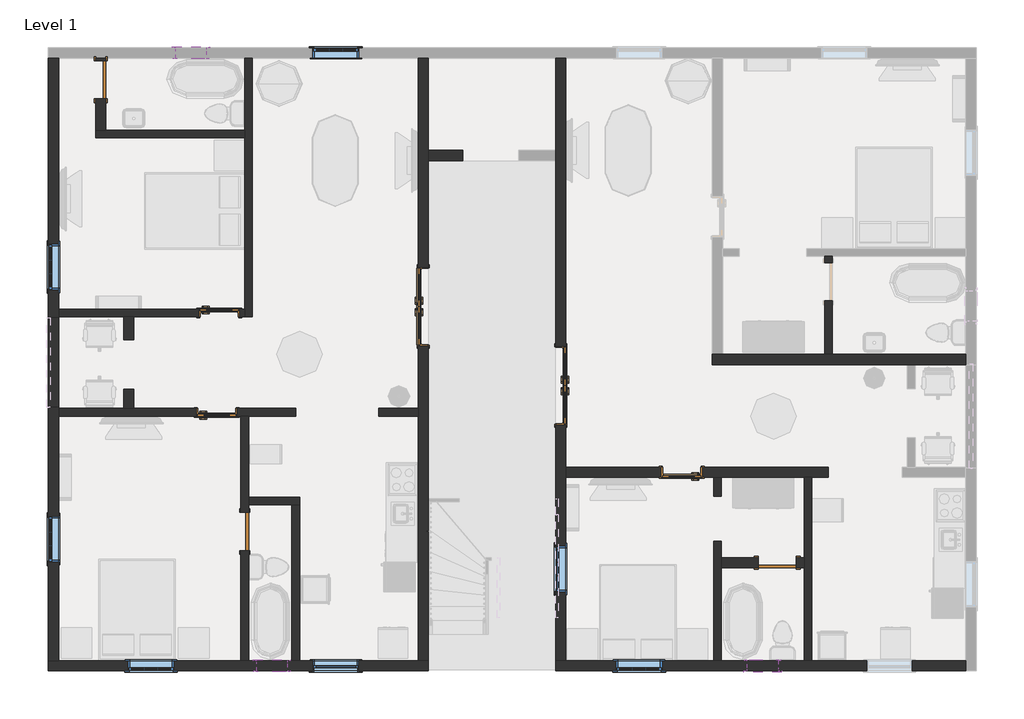
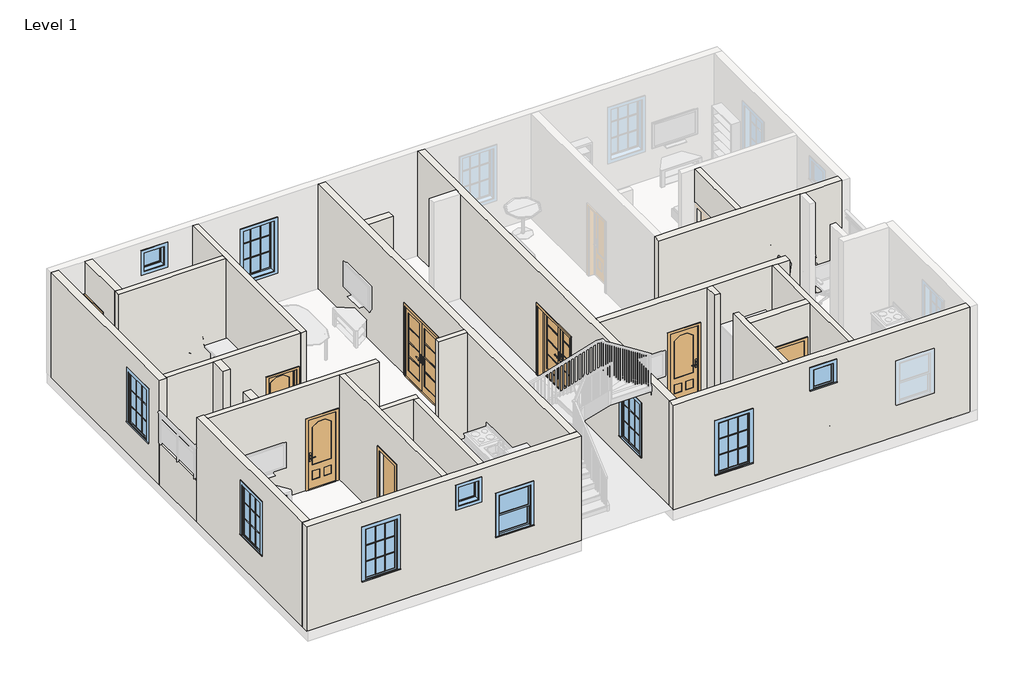
# One storey, part 1 of 4: 26 walls, 10 windows, 8 doors.
"""IFC4 building model written with IfcOpenShell, lengths in millimetres."""

from ifc_helpers import new_model, si_unit, frame, origin, origin_with_axes, place, context, project, spatial, polyline, outline, extrude, faceted_brep, transform, mapped, element, save
from components import door_4b146b56, door_14b9be53, door_41326d50, door_b03bd389, door_53b1b562, door_255cab33, window_58e1470a, window_31198920, window_e41d21a6

model = new_model("IFC4")

# Units and contexts
model_context = context("Model", 3, world=origin())
ifc_project = project(units=[si_unit("LENGTHUNIT", "METRE", prefix="MILLI")], contexts=[model_context])

# Site, building, storey
site = spatial("IfcSite", under=ifc_project)
building = spatial("IfcBuilding", under=site)
storey = spatial("IfcBuildingStorey", under=building, Name="Level 1", Elevation=0.0)

# Doors
placement = place(None, origin())
door_shape = door_4b146b56(model_context)
element("IfcDoor", 1, ObjectType="30\" x 80\"", at=placement, inside=storey, context=model_context, shape_type="MappedRepresentation", body=[
    mapped(door_shape, transform((-13233.5808972, 7613.5673354, 0.0), x_axis=(-1.0, 0.0, 0.0), y_axis=(0.0, -1.0, 0.0), z_axis=(0.0, 0.0, 1.0))),
])
door_2_shape = door_14b9be53(model_context)
element("IfcDoor", 2, ObjectType="30\" x 80\"", at=placement, inside=storey, context=model_context, shape_type="MappedRepresentation", body=[
    mapped(door_2_shape, transform((-13284.3808972, 5626.0173354, 0.0), x_axis=(-1.0, 0.0, 0.0), y_axis=(0.0, -1.0, 0.0), z_axis=(0.0, 0.0, 1.0))),
])
door_3_shape = door_41326d50(model_context)
element("IfcDoor", 3, ObjectType="30\" x 80\"", at=placement, inside=storey, context=model_context, shape_type="MappedRepresentation", body=[
    mapped(door_3_shape, transform((-4013.3808972, 4432.2173354, 0.0), x_axis=(1.0, 0.0, 0.0), y_axis=(0.0, 1.0, 0.0), z_axis=(0.0, 0.0, 1.0))),
])
door_4_shape = door_b03bd389(model_context)
element("IfcDoor", 4, ObjectType="Door-Exterior-Double-Full Glass-Wood_Clad : 60\" x 80\"", at=placement, inside=storey, context=model_context, shape_type="MappedRepresentation", body=[
    mapped(door_4_shape, transform((-9172.7558972, 7737.3923354, 0.0), x_axis=(0.0, 1.0, 0.0), y_axis=(-1.0, 0.0, 0.0), z_axis=(0.0, 0.0, 1.0))),
])
element("IfcDoor", 5, ObjectType="Door-Exterior-Double-Full Glass-Wood_Clad : 60\" x 80\"", at=placement, inside=storey, context=model_context, shape_type="MappedRepresentation", body=[
    mapped(door_4_shape, transform((-6423.2058972, 6162.5923354, 0.0), x_axis=(0.0, -1.0, 0.0), y_axis=(1.0, 0.0, 0.0), z_axis=(0.0, 0.0, 1.0))),
])
door_5_shape = door_53b1b562(model_context)
element("IfcDoor", 6, ObjectType="Single-Flush : 30\" x 80\"", at=placement, inside=storey, context=model_context, shape_type="MappedRepresentation", body=[
    mapped(door_5_shape, transform((-15595.7808972, 12258.5923354, 0.0), x_axis=(0.0, 1.0, 0.0), y_axis=(-1.0, 0.0, 0.0), z_axis=(0.0, 0.0, 1.0))),
])
element("IfcDoor", 7, ObjectType="Single-Flush : 30\" x 80\"", at=placement, inside=storey, context=model_context, shape_type="MappedRepresentation", body=[
    mapped(door_5_shape, transform((-2108.3808972, 2631.9923354, 0.0), x_axis=(1.0, 0.0, 0.0), y_axis=(0.0, 1.0, 0.0), z_axis=(0.0, 0.0, 1.0))),
])
door_6_shape = door_255cab33(model_context)
element("IfcDoor", 8, ObjectType="Single-Flush : 30\" x 80\"", at=placement, inside=storey, context=model_context, shape_type="MappedRepresentation", body=[
    mapped(door_6_shape, transform((-12725.5808972, 3254.2923354, 0.0), x_axis=(0.0, 1.0, 0.0), y_axis=(-1.0, 0.0, 0.0), z_axis=(0.0, 0.0, 1.0))),
])

# Walls
element("IfcWall", 9, ObjectType="Generic - 8\"", at=placement, inside=storey, context=model_context, shape_type="Brep", body=[
    faceted_brep([(1650.8191028, 676.1923354, 0.0), (-1422.5808972, 676.1923354, 0.0), (-1574.9808972, 676.1923354, 0.0), (-3225.9808972, 676.1923354, 0.0), (-3378.3808972, 676.1923354, 0.0), (-6324.7808972, 676.1923354, 0.0), (-6527.9808972, 676.1923354, 0.0), (-6527.9808972, 676.1923354, 3048.0), (-6324.7808972, 676.1923354, 3048.0), (-3378.3808972, 676.1923354, 3048.0), (-3225.9808972, 676.1923354, 3048.0), (-1574.9808972, 676.1923354, 3048.0), (-1422.5808972, 676.1923354, 3048.0), (1650.8191028, 676.1923354, 3048.0), (-330.3808972, 676.1923354, 2133.6), (-330.3808972, 676.1923354, 914.4), (584.0191028, 676.1923354, 914.4), (584.0191028, 676.1923354, 2133.6), (-5321.4808972, 676.1923354, 2133.6), (-5321.4808972, 676.1923354, 609.6), (-4407.0808972, 676.1923354, 609.6), (-4407.0808972, 676.1923354, 2133.6), (-2705.2808972, 676.1923354, 2768.6), (-2705.2808972, 676.1923354, 2159.0), (-2095.6808972, 676.1923354, 2159.0), (-2095.6808972, 676.1923354, 2768.6), (1650.8191028, 472.9923354, 0.0), (1650.8191028, 472.9923354, 3048.0), (-6527.9808972, 472.9923354, 3048.0), (-6527.9808972, 472.9923354, 0.0), (-330.3808972, 472.9923354, 2133.6), (584.0191028, 472.9923354, 2133.6), (584.0191028, 472.9923354, 914.4), (-330.3808972, 472.9923354, 914.4), (-5321.4808972, 472.9923354, 2133.6), (-4407.0808972, 472.9923354, 2133.6), (-4407.0808972, 472.9923354, 609.6), (-5321.4808972, 472.9923354, 609.6), (-2705.2808972, 472.9923354, 2768.6), (-2095.6808972, 472.9923354, 2768.6), (-2095.6808972, 472.9923354, 2159.0), (-2705.2808972, 472.9923354, 2159.0)], [[[0, 1, 2, 3, 4, 5, 6, 7, 8, 9, 10, 11, 12, 13], [14, 15, 16, 17], [18, 19, 20, 21], [22, 23, 24, 25]], [[26, 27, 28, 29], [30, 31, 32, 33], [34, 35, 36, 37], [38, 39, 40, 41]], [[6, 5, 4, 3, 2, 1, 0, 26, 29]], [[13, 12, 11, 10, 9, 8, 7, 28, 27]], [[0, 13, 27, 26]], [[7, 6, 29, 28]], [[15, 14, 30, 33]], [[16, 15, 33, 32]], [[17, 16, 32, 31]], [[14, 17, 31, 30]], [[19, 18, 34, 37]], [[20, 19, 37, 36]], [[21, 20, 36, 35]], [[18, 21, 35, 34]], [[23, 22, 38, 41]], [[24, 23, 41, 40]], [[25, 24, 40, 39]], [[22, 25, 39, 38]]]),
])
element("IfcWall", 10, ObjectType="Generic - 8\"", at=placement, inside=storey, context=model_context, shape_type="Brep", body=[
    faceted_brep([(-16433.9808972, 676.1923354, 0.0), (-16433.9808972, 5552.9923354, 0.0), (-16433.9808972, 5705.3923354, 0.0), (-16433.9808972, 5730.7923354, 0.0), (-16433.9808972, 5730.7923354, 1219.2), (-16433.9808972, 5730.7923354, 3048.0), (-16433.9808972, 5705.3923354, 3048.0), (-16433.9808972, 5552.9923354, 3048.0), (-16433.9808972, 676.1923354, 3048.0), (-16433.9808972, 3559.0923354, 2438.4), (-16433.9808972, 3559.0923354, 914.4), (-16433.9808972, 2644.6923354, 914.4), (-16433.9808972, 2644.6923354, 2438.4), (-16637.1808972, 676.1923354, 0.0), (-16637.1808972, 676.1923354, 3048.0), (-16637.1808972, 5730.7923354, 3048.0), (-16637.1808972, 5730.7923354, 1219.2), (-16637.1808972, 5730.7923354, 0.0), (-16637.1808972, 3559.0923354, 2438.4), (-16637.1808972, 2644.6923354, 2438.4), (-16637.1808972, 2644.6923354, 914.4), (-16637.1808972, 3559.0923354, 914.4)], [[[0, 1, 2, 3, 4, 5, 6, 7, 8], [9, 10, 11, 12]], [[13, 14, 15, 16, 17], [18, 19, 20, 21]], [[3, 2, 1, 0, 13, 17]], [[5, 4, 3, 17, 16, 15]], [[8, 7, 6, 5, 15, 14]], [[0, 8, 14, 13]], [[10, 9, 18, 21]], [[11, 10, 21, 20]], [[12, 11, 20, 19]], [[9, 12, 19, 18]]]),
])
element("IfcWall", 11, ObjectType="Generic - 8\"", at=placement, inside=storey, context=model_context, shape_type="Brep", body=[
    faceted_brep([(-6527.9808972, 676.1923354, 3048.0), (-6527.9808972, 10645.6923354, 3048.0), (-6527.9808972, 10848.8923354, 3048.0), (-6527.9808972, 12690.3923354, 3048.0), (-6527.9808972, 12690.3923354, 0.0), (-6527.9808972, 10848.8923354, 0.0), (-6527.9808972, 10645.6923354, 0.0), (-6527.9808972, 6949.9923354, 0.0), (-6527.9808972, 6949.9923354, 2057.4), (-6527.9808972, 5375.1923354, 2057.4), (-6527.9808972, 5375.1923354, 0.0), (-6527.9808972, 676.1923354, 0.0), (-6527.9808972, 2962.1923354, 2133.6), (-6527.9808972, 2047.7923354, 2133.6), (-6527.9808972, 2047.7923354, 609.6), (-6527.9808972, 2962.1923354, 609.6), (-6324.7808972, 12690.3923354, 3048.0), (-6324.7808972, 4536.9923354, 3048.0), (-6324.7808972, 4333.7923354, 3048.0), (-6324.7808972, 676.1923354, 3048.0), (-6324.7808972, 676.1923354, 0.0), (-6324.7808972, 4333.7923354, 0.0), (-6324.7808972, 4536.9923354, 0.0), (-6324.7808972, 5375.1923354, 0.0), (-6324.7808972, 5375.1923354, 2057.4), (-6324.7808972, 6949.9923354, 2057.4), (-6324.7808972, 6949.9923354, 0.0), (-6324.7808972, 12690.3923354, 0.0), (-6324.7808972, 2962.1923354, 2133.6), (-6324.7808972, 2962.1923354, 609.6), (-6324.7808972, 2047.7923354, 609.6), (-6324.7808972, 2047.7923354, 2133.6)], [[[0, 1, 2, 3, 4, 5, 6, 7, 8, 9, 10, 11], [12, 13, 14, 15]], [[16, 17, 18, 19, 20, 21, 22, 23, 24, 25, 26, 27], [28, 29, 30, 31]], [[4, 27, 26, 7, 6, 5]], [[20, 11, 10, 23, 22, 21]], [[3, 2, 1, 0, 19, 18, 17, 16]], [[4, 3, 16, 27]], [[0, 11, 20, 19]], [[9, 24, 23, 10]], [[24, 9, 8, 25]], [[25, 8, 7, 26]], [[29, 28, 12, 15]], [[30, 29, 15, 14]], [[31, 30, 14, 13]], [[28, 31, 13, 12]]]),
])
element("IfcWall", 12, ObjectType="Generic - 8\"", at=placement, inside=storey, context=model_context, shape_type="Brep", body=[
    faceted_brep([(-9271.1808972, 676.1923354, 3048.0), (-9271.1808972, 5552.9923354, 3048.0), (-9271.1808972, 5705.3923354, 3048.0), (-9271.1808972, 12690.3923354, 3048.0), (-9271.1808972, 12690.3923354, 0.0), (-9271.1808972, 8524.7923354, 0.0), (-9271.1808972, 8524.7923354, 2057.4), (-9271.1808972, 6949.9923354, 2057.4), (-9271.1808972, 6949.9923354, 0.0), (-9271.1808972, 5705.3923354, 0.0), (-9271.1808972, 5552.9923354, 0.0), (-9271.1808972, 676.1923354, 0.0), (-9067.9808972, 12690.3923354, 3048.0), (-9067.9808972, 10848.8923354, 3048.0), (-9067.9808972, 10645.6923354, 3048.0), (-9067.9808972, 676.1923354, 3048.0), (-9067.9808972, 676.1923354, 0.0), (-9067.9808972, 6949.9923354, 0.0), (-9067.9808972, 6949.9923354, 2057.4), (-9067.9808972, 8524.7923354, 2057.4), (-9067.9808972, 8524.7923354, 0.0), (-9067.9808972, 10645.6923354, 0.0), (-9067.9808972, 10848.8923354, 0.0), (-9067.9808972, 12690.3923354, 0.0)], [[[0, 1, 2, 3, 4, 5, 6, 7, 8, 9, 10, 11]], [[12, 13, 14, 15, 16, 17, 18, 19, 20, 21, 22, 23]], [[4, 23, 22, 21, 20, 5]], [[16, 11, 10, 9, 8, 17]], [[3, 2, 1, 0, 15, 14, 13, 12]], [[4, 3, 12, 23]], [[0, 11, 16, 15]], [[19, 6, 5, 20]], [[6, 19, 18, 7]], [[7, 18, 17, 8]]]),
])
element("IfcWall", 13, ObjectType="Generic - 8\"", at=placement, inside=storey, context=model_context, shape_type="Brep", body=[
    faceted_brep([(-1092.3808972, 4333.7923354, 0.0), (-1092.3808972, 4333.7923354, 3048.0), (-1422.5808972, 4333.7923354, 3048.0), (-1574.9808972, 4333.7923354, 3048.0), (-3225.9808972, 4333.7923354, 3048.0), (-3378.3808972, 4333.7923354, 3048.0), (-6324.7808972, 4333.7923354, 3048.0), (-6324.7808972, 4333.7923354, 0.0), (-4419.7808972, 4333.7923354, 0.0), (-4419.7808972, 4333.7923354, 2057.4), (-3606.9808972, 4333.7923354, 2057.4), (-3606.9808972, 4333.7923354, 0.0), (-3378.3808972, 4333.7923354, 0.0), (-3225.9808972, 4333.7923354, 0.0), (-1574.9808972, 4333.7923354, 0.0), (-1422.5808972, 4333.7923354, 0.0), (-1092.3808972, 4536.9923354, 3048.0), (-1092.3808972, 4536.9923354, 0.0), (-3606.9808972, 4536.9923354, 0.0), (-3606.9808972, 4536.9923354, 2057.4), (-4419.7808972, 4536.9923354, 2057.4), (-4419.7808972, 4536.9923354, 0.0), (-6324.7808972, 4536.9923354, 0.0), (-6324.7808972, 4536.9923354, 3048.0)], [[[0, 1, 2, 3, 4, 5, 6, 7, 8, 9, 10, 11, 12, 13, 14, 15]], [[16, 17, 18, 19, 20, 21, 22, 23]], [[17, 0, 15, 14, 13, 12, 11, 18]], [[7, 22, 21, 8]], [[1, 0, 17, 16]], [[6, 5, 4, 3, 2, 1, 16, 23]], [[7, 6, 23, 22]], [[10, 19, 18, 11]], [[19, 10, 9, 20]], [[20, 9, 8, 21]]]),
])
element("IfcWall", 14, ObjectType="Generic - 8\"", at=placement, inside=storey, context=model_context, shape_type="Brep", body=[
    faceted_brep([(1650.8191028, 6784.8923354, 0.0), (-1016.1808972, 6784.8923354, 0.0), (-1168.5808972, 6784.8923354, 0.0), (-3200.5808972, 6784.8923354, 0.0), (-3403.7808972, 6784.8923354, 0.0), (-3403.7808972, 6784.8923354, 3048.0), (-3200.5808972, 6784.8923354, 3048.0), (-1168.5808972, 6784.8923354, 3048.0), (-1016.1808972, 6784.8923354, 3048.0), (1650.8191028, 6784.8923354, 3048.0), (1650.8191028, 6581.6923354, 0.0), (1650.8191028, 6581.6923354, 3048.0), (634.8191028, 6581.6923354, 3048.0), (482.4191028, 6581.6923354, 3048.0), (-3403.7808972, 6581.6923354, 3048.0), (-3403.7808972, 6581.6923354, 0.0), (482.4191028, 6581.6923354, 0.0), (634.8191028, 6581.6923354, 0.0)], [[[0, 1, 2, 3, 4, 5, 6, 7, 8, 9]], [[10, 11, 12, 13, 14, 15, 16, 17]], [[4, 3, 2, 1, 0, 10, 17, 16, 15]], [[9, 8, 7, 6, 5, 14, 13, 12, 11]], [[0, 9, 11, 10]], [[5, 4, 15, 14]]]),
])
element("IfcWall", 15, ObjectType="Generic - 8\"", at=placement, inside=storey, context=model_context, shape_type="SweptSolid", body=[
    extrude(outline(polyline([(-8382.1808972, 10645.6923354), (-9067.9808972, 10645.6923354), (-9067.9808972, 10848.8923354), (-8382.1808972, 10848.8923354), (-8382.1808972, 10645.6923354)])), origin_with_axes(), (0.0, 0.0, 1.0), 3048.0),
])
element("IfcWall", 16, ObjectType="Generic - 8\"", at=placement, inside=storey, context=model_context, shape_type="Brep", body=[
    faceted_brep([(-9067.9808972, 676.1923354, 0.0), (-9271.1808972, 676.1923354, 0.0), (-11633.3808972, 676.1923354, 0.0), (-11785.7808972, 676.1923354, 0.0), (-12649.3808972, 676.1923354, 0.0), (-12801.7808972, 676.1923354, 0.0), (-16433.9808972, 676.1923354, 0.0), (-16637.1808972, 676.1923354, 0.0), (-16637.1808972, 676.1923354, 3048.0), (-16433.9808972, 676.1923354, 3048.0), (-12801.7808972, 676.1923354, 3048.0), (-12649.3808972, 676.1923354, 3048.0), (-11785.7808972, 676.1923354, 3048.0), (-11633.3808972, 676.1923354, 3048.0), (-9271.1808972, 676.1923354, 3048.0), (-9067.9808972, 676.1923354, 3048.0), (-15049.6808972, 676.1923354, 2438.4), (-15049.6808972, 676.1923354, 914.4), (-14135.2808972, 676.1923354, 914.4), (-14135.2808972, 676.1923354, 2438.4), (-11366.6808972, 676.1923354, 2133.6), (-11366.6808972, 676.1923354, 914.4), (-10452.2808972, 676.1923354, 914.4), (-10452.2808972, 676.1923354, 2133.6), (-11874.6808972, 676.1923354, 2768.6), (-12484.2808972, 676.1923354, 2768.6), (-12484.2808972, 676.1923354, 2159.0), (-11874.6808972, 676.1923354, 2159.0), (-9067.9808972, 472.9923354, 0.0), (-9067.9808972, 472.9923354, 3048.0), (-16637.1808972, 472.9923354, 3048.0), (-16637.1808972, 472.9923354, 0.0), (-15049.6808972, 472.9923354, 2438.4), (-14135.2808972, 472.9923354, 2438.4), (-14135.2808972, 472.9923354, 914.4), (-15049.6808972, 472.9923354, 914.4), (-11366.6808972, 472.9923354, 2133.6), (-10452.2808972, 472.9923354, 2133.6), (-10452.2808972, 472.9923354, 914.4), (-11366.6808972, 472.9923354, 914.4), (-11874.6808972, 472.9923354, 2768.6), (-11874.6808972, 472.9923354, 2159.0), (-12484.2808972, 472.9923354, 2159.0), (-12484.2808972, 472.9923354, 2768.6)], [[[0, 1, 2, 3, 4, 5, 6, 7, 8, 9, 10, 11, 12, 13, 14, 15], [16, 17, 18, 19], [20, 21, 22, 23], [24, 25, 26, 27]], [[28, 29, 30, 31], [32, 33, 34, 35], [36, 37, 38, 39], [40, 41, 42, 43]], [[7, 6, 5, 4, 3, 2, 1, 0, 28, 31]], [[15, 14, 13, 12, 11, 10, 9, 8, 30, 29]], [[8, 7, 31, 30]], [[0, 15, 29, 28]], [[17, 16, 32, 35]], [[18, 17, 35, 34]], [[19, 18, 34, 33]], [[16, 19, 33, 32]], [[21, 20, 36, 39]], [[22, 21, 39, 38]], [[23, 22, 38, 37]], [[20, 23, 37, 36]], [[41, 40, 24, 27]], [[42, 41, 27, 26]], [[43, 42, 26, 25]], [[40, 43, 25, 24]]]),
])
element("IfcWall", 17, ObjectType="Generic - 8\"", at=placement, inside=storey, context=model_context, shape_type="SweptSolid", body=[
    extrude(outline(polyline([(12690.3923354, 0.0), (12639.5923354, 0.0), (12639.5923354, 2032.0), (11877.5923354, 2032.0), (11877.5923354, 0.0), (11255.2923354, 0.0), (11255.2923354, 3048.0), (12690.3923354, 3048.0), (12690.3923354, 0.0)])), frame((-15697.3808972, 0.0, 0.0), z_axis=(1.0, 0.0, 0.0), x_axis=(0.0, 1.0, 0.0)), (0.0, 0.0, 1.0), 203.2),
])
element("IfcWall", 18, ObjectType="Generic - 8\"", at=placement, inside=storey, context=model_context, shape_type="SweptSolid", body=[
    extrude(outline(polyline([(2032.0, -1727.3808972), (0.0, -1727.3808972), (0.0, -1574.9808972), (3048.0, -1574.9808972), (3048.0, -3225.9808972), (0.0, -3225.9808972), (0.0, -2489.3808972), (2032.0, -2489.3808972), (2032.0, -1727.3808972)])), frame((0.0, 2530.3923354, 0.0), z_axis=(0.0, 1.0, 0.0), x_axis=(0.0, 0.0, 1.0)), (0.0, 0.0, 1.0), 203.2),
])
element("IfcWall", 19, ObjectType="Generic - 8\"", at=placement, inside=storey, context=model_context, shape_type="SweptSolid", body=[
    extrude(outline(polyline([(-15138.5808972, 7076.9923354), (-15138.5808972, 7534.1923354), (-14935.3808972, 7534.1923354), (-14935.3808972, 7076.9923354), (-15138.5808972, 7076.9923354)])), origin_with_axes(), (0.0, 0.0, 1.0), 3048.0),
])
element("IfcWall", 20, ObjectType="Generic - 8\"", at=placement, inside=storey, context=model_context, shape_type="SweptSolid", body=[
    extrude(outline(polyline([(-15138.5808972, 5705.3923354), (-15138.5808972, 6086.3923354), (-14935.3808972, 6086.3923354), (-14935.3808972, 5705.3923354), (-15138.5808972, 5705.3923354)])), origin_with_axes(), (0.0, 0.0, 1.0), 3048.0),
])
element("IfcWall", 21, ObjectType="Generic - 8\"", at=placement, inside=storey, context=model_context, shape_type="Brep", body=[
    faceted_brep([(-16433.9808972, 7508.7923354, 0.0), (-16433.9808972, 7534.1923354, 0.0), (-16433.9808972, 7686.5923354, 0.0), (-16433.9808972, 12690.3923354, 0.0), (-16433.9808972, 12690.3923354, 3048.0), (-16433.9808972, 7686.5923354, 3048.0), (-16433.9808972, 7534.1923354, 3048.0), (-16433.9808972, 7508.7923354, 3048.0), (-16433.9808972, 7508.7923354, 1219.2), (-16433.9808972, 8981.9923354, 2438.4), (-16433.9808972, 8981.9923354, 914.4), (-16433.9808972, 8067.5923354, 914.4), (-16433.9808972, 8067.5923354, 2438.4), (-16637.1808972, 7508.7923354, 0.0), (-16637.1808972, 7508.7923354, 1219.2), (-16637.1808972, 7508.7923354, 3048.0), (-16637.1808972, 12690.3923354, 3048.0), (-16637.1808972, 12690.3923354, 0.0), (-16637.1808972, 8981.9923354, 2438.4), (-16637.1808972, 8067.5923354, 2438.4), (-16637.1808972, 8067.5923354, 914.4), (-16637.1808972, 8981.9923354, 914.4)], [[[0, 1, 2, 3, 4, 5, 6, 7, 8], [9, 10, 11, 12]], [[13, 14, 15, 16, 17], [18, 19, 20, 21]], [[3, 2, 1, 0, 13, 17]], [[7, 6, 5, 4, 16, 15]], [[0, 8, 7, 15, 14, 13]], [[4, 3, 17, 16]], [[10, 9, 18, 21]], [[11, 10, 21, 20]], [[12, 11, 20, 19]], [[9, 12, 19, 18]]]),
])
element("IfcWall", 22, ObjectType="Generic - 8\"", at=placement, inside=storey, context=model_context, shape_type="SweptSolid", body=[
    extrude(outline(polyline([(-16433.9808972, 7508.7923354), (-16433.9808972, 5730.7923354), (-16637.1808972, 5730.7923354), (-16637.1808972, 7508.7923354), (-16433.9808972, 7508.7923354)])), origin_with_axes(), (0.0, 0.0, 1.0), 1219.2),
])
element("IfcWall", 23, ObjectType="INNER", at=placement, inside=storey, context=model_context, shape_type="Brep", body=[
    faceted_brep([(-12725.5808972, 12690.3923354, 0.0), (-12725.5808972, 11255.2923354, 0.0), (-12725.5808972, 11102.8923354, 0.0), (-12725.5808972, 7686.5923354, 0.0), (-12725.5808972, 7534.1923354, 0.0), (-12725.5808972, 7534.1923354, 3048.0), (-12725.5808972, 7686.5923354, 3048.0), (-12725.5808972, 11102.8923354, 3048.0), (-12725.5808972, 11255.2923354, 3048.0), (-12725.5808972, 12690.3923354, 3048.0), (-12573.1808972, 12690.3923354, 0.0), (-12573.1808972, 12690.3923354, 3048.0), (-12573.1808972, 7534.1923354, 3048.0), (-12573.1808972, 7534.1923354, 0.0)], [[[0, 1, 2, 3, 4, 5, 6, 7, 8, 9]], [[10, 11, 12, 13]], [[4, 3, 2, 1, 0, 10, 13]], [[9, 8, 7, 6, 5, 12, 11]], [[0, 9, 11, 10]], [[5, 4, 13, 12]]]),
])
element("IfcWall", 24, ObjectType="INNER", at=placement, inside=storey, context=model_context, shape_type="SweptSolid", body=[
    extrude(outline(polyline([(-10058.5808972, 5705.3923354), (-9271.1808972, 5705.3923354), (-9271.1808972, 5552.9923354), (-10058.5808972, 5552.9923354), (-10058.5808972, 5705.3923354)])), origin_with_axes(), (0.0, 0.0, 1.0), 3048.0),
])
element("IfcWall", 25, ObjectType="INNER", at=placement, inside=storey, context=model_context, shape_type="Brep", body=[
    faceted_brep([(-12725.5808972, 7534.1923354, 3048.0), (-14935.3808972, 7534.1923354, 3048.0), (-15138.5808972, 7534.1923354, 3048.0), (-16433.9808972, 7534.1923354, 3048.0), (-16433.9808972, 7534.1923354, 0.0), (-15138.5808972, 7534.1923354, 0.0), (-14935.3808972, 7534.1923354, 0.0), (-13639.9808972, 7534.1923354, 0.0), (-13639.9808972, 7534.1923354, 2057.4), (-12827.1808972, 7534.1923354, 2057.4), (-12827.1808972, 7534.1923354, 0.0), (-12725.5808972, 7534.1923354, 0.0), (-16433.9808972, 7686.5923354, 3048.0), (-12725.5808972, 7686.5923354, 3048.0), (-12725.5808972, 7686.5923354, 0.0), (-12827.1808972, 7686.5923354, 0.0), (-12827.1808972, 7686.5923354, 2057.4), (-13639.9808972, 7686.5923354, 2057.4), (-13639.9808972, 7686.5923354, 0.0), (-16433.9808972, 7686.5923354, 0.0)], [[[0, 1, 2, 3, 4, 5, 6, 7, 8, 9, 10, 11]], [[12, 13, 14, 15, 16, 17, 18, 19]], [[4, 19, 18, 7, 6, 5]], [[14, 11, 10, 15]], [[3, 2, 1, 0, 13, 12]], [[4, 3, 12, 19]], [[0, 11, 14, 13]], [[17, 8, 7, 18]], [[8, 17, 16, 9]], [[9, 16, 15, 10]]]),
])
element("IfcWall", 26, ObjectType="INNER", at=placement, inside=storey, context=model_context, shape_type="Brep", body=[
    faceted_brep([(-12801.7808972, 5552.9923354, 0.0), (-12801.7808972, 3635.2923354, 0.0), (-12801.7808972, 3635.2923354, 2032.0), (-12801.7808972, 2873.2923354, 2032.0), (-12801.7808972, 2873.2923354, 0.0), (-12801.7808972, 676.1923354, 0.0), (-12801.7808972, 676.1923354, 3048.0), (-12801.7808972, 5552.9923354, 3048.0), (-12649.3808972, 3635.2923354, 2032.0), (-12649.3808972, 3635.2923354, 0.0), (-12649.3808972, 3787.6923354, 0.0), (-12649.3808972, 3940.0923354, 0.0), (-12649.3808972, 5552.9923354, 0.0), (-12649.3808972, 5552.9923354, 3048.0), (-12649.3808972, 3940.0923354, 3048.0), (-12649.3808972, 3787.6923354, 3048.0), (-12649.3808972, 676.1923354, 3048.0), (-12649.3808972, 676.1923354, 0.0), (-12649.3808972, 2873.2923354, 0.0), (-12649.3808972, 2873.2923354, 2032.0)], [[[0, 1, 2, 3, 4, 5, 6, 7]], [[8, 9, 10, 11, 12, 13, 14, 15, 16, 17, 18, 19]], [[18, 17, 5, 4]], [[12, 11, 10, 9, 1, 0]], [[7, 6, 16, 15, 14, 13]], [[6, 5, 17, 16]], [[0, 7, 13, 12]], [[2, 1, 9, 8]], [[3, 2, 8, 19]], [[4, 3, 19, 18]]]),
])
element("IfcWall", 27, ObjectType="INNER", at=placement, inside=storey, context=model_context, shape_type="Brep", body=[
    faceted_brep([(-16433.9808972, 5705.3923354, 3048.0), (-15138.5808972, 5705.3923354, 3048.0), (-14935.3808972, 5705.3923354, 3048.0), (-11709.5808972, 5705.3923354, 3048.0), (-11709.5808972, 5705.3923354, 0.0), (-12877.9808972, 5705.3923354, 0.0), (-12877.9808972, 5705.3923354, 2057.4), (-13690.7808972, 5705.3923354, 2057.4), (-13690.7808972, 5705.3923354, 0.0), (-14935.3808972, 5705.3923354, 0.0), (-15138.5808972, 5705.3923354, 0.0), (-16433.9808972, 5705.3923354, 0.0), (-11709.5808972, 5552.9923354, 3048.0), (-12649.3808972, 5552.9923354, 3048.0), (-12801.7808972, 5552.9923354, 3048.0), (-16433.9808972, 5552.9923354, 3048.0), (-16433.9808972, 5552.9923354, 0.0), (-13690.7808972, 5552.9923354, 0.0), (-13690.7808972, 5552.9923354, 2057.4), (-12877.9808972, 5552.9923354, 2057.4), (-12877.9808972, 5552.9923354, 0.0), (-12801.7808972, 5552.9923354, 0.0), (-12649.3808972, 5552.9923354, 0.0), (-11709.5808972, 5552.9923354, 0.0)], [[[0, 1, 2, 3, 4, 5, 6, 7, 8, 9, 10, 11]], [[12, 13, 14, 15, 16, 17, 18, 19, 20, 21, 22, 23]], [[4, 23, 22, 21, 20, 5]], [[16, 11, 10, 9, 8, 17]], [[3, 2, 1, 0, 15, 14, 13, 12]], [[4, 3, 12, 23]], [[0, 11, 16, 15]], [[7, 18, 17, 8]], [[18, 7, 6, 19]], [[19, 6, 5, 20]]]),
])
element("IfcWall", 28, ObjectType="INNER", at=placement, inside=storey, context=model_context, shape_type="Brep", body=[
    faceted_brep([(-1574.9808972, 4333.7923354, 0.0), (-1574.9808972, 2733.5923354, 0.0), (-1574.9808972, 2530.3923354, 0.0), (-1574.9808972, 676.1923354, 0.0), (-1574.9808972, 676.1923354, 3048.0), (-1574.9808972, 2530.3923354, 3048.0), (-1574.9808972, 2733.5923354, 3048.0), (-1574.9808972, 4333.7923354, 3048.0), (-1422.5808972, 4333.7923354, 0.0), (-1422.5808972, 4333.7923354, 3048.0), (-1422.5808972, 676.1923354, 3048.0), (-1422.5808972, 676.1923354, 0.0)], [[[0, 1, 2, 3, 4, 5, 6, 7]], [[8, 9, 10, 11]], [[3, 2, 1, 0, 8, 11]], [[7, 6, 5, 4, 10, 9]], [[4, 3, 11, 10]], [[0, 7, 9, 8]]]),
])
element("IfcWall", 29, ObjectType="INNER", at=placement, inside=storey, context=model_context, shape_type="Brep", body=[
    faceted_brep([(-3225.9808972, 676.1923354, 0.0), (-3225.9808972, 2530.3923354, 0.0), (-3225.9808972, 2733.5923354, 0.0), (-3225.9808972, 3063.7923354, 0.0), (-3225.9808972, 3063.7923354, 3048.0), (-3225.9808972, 2733.5923354, 3048.0), (-3225.9808972, 2530.3923354, 3048.0), (-3225.9808972, 676.1923354, 3048.0), (-3378.3808972, 676.1923354, 0.0), (-3378.3808972, 676.1923354, 3048.0), (-3378.3808972, 3063.7923354, 3048.0), (-3378.3808972, 3063.7923354, 0.0)], [[[0, 1, 2, 3, 4, 5, 6, 7]], [[8, 9, 10, 11]], [[3, 2, 1, 0, 8, 11]], [[4, 3, 11, 10]], [[7, 6, 5, 4, 10, 9]], [[0, 7, 9, 8]]]),
])
element("IfcWall", 30, ObjectType="INNER", at=placement, inside=storey, context=model_context, shape_type="SweptSolid", body=[
    extrude(outline(polyline([(8740.6923354, 0.0), (8613.6923354, 0.0), (8613.6923354, 2032.0), (7851.6923354, 2032.0), (7851.6923354, 0.0), (6784.8923354, 0.0), (6784.8923354, 3048.0), (8740.6923354, 3048.0), (8740.6923354, 0.0)])), frame((-1168.5808972, 0.0, 0.0), z_axis=(1.0, 0.0, 0.0), x_axis=(0.0, 1.0, 0.0)), (0.0, 0.0, 1.0), 152.4),
])
element("IfcWall", 31, ObjectType="INNER", at=placement, inside=storey, context=model_context, shape_type="SweptSolid", body=[
    extrude(outline(polyline([(-3225.9808972, 4333.7923354), (-3225.9808972, 3952.7923354), (-3378.3808972, 3952.7923354), (-3378.3808972, 4333.7923354), (-3225.9808972, 4333.7923354)])), origin_with_axes(), (0.0, 0.0, 1.0), 3048.0),
])
element("IfcWall", 32, ObjectType="INNER", at=placement, inside=storey, context=model_context, shape_type="Brep", body=[
    faceted_brep([(-12725.5808972, 11255.2923354, 0.0), (-15494.1808972, 11255.2923354, 0.0), (-15697.3808972, 11255.2923354, 0.0), (-15697.3808972, 11255.2923354, 3048.0), (-15494.1808972, 11255.2923354, 3048.0), (-12725.5808972, 11255.2923354, 3048.0), (-12725.5808972, 11102.8923354, 0.0), (-12725.5808972, 11102.8923354, 3048.0), (-15697.3808972, 11102.8923354, 3048.0), (-15697.3808972, 11102.8923354, 0.0)], [[[0, 1, 2, 3, 4, 5]], [[6, 7, 8, 9]], [[2, 1, 0, 6, 9]], [[5, 4, 3, 8, 7]], [[0, 5, 7, 6]], [[3, 2, 9, 8]]]),
])
element("IfcWall", 33, ObjectType="INNER", at=placement, inside=storey, context=model_context, shape_type="Brep", body=[
    faceted_brep([(-12649.3808972, 3787.6923354, 0.0), (-11785.7808972, 3787.6923354, 0.0), (-11633.3808972, 3787.6923354, 0.0), (-11633.3808972, 3787.6923354, 3048.0), (-11785.7808972, 3787.6923354, 3048.0), (-12649.3808972, 3787.6923354, 3048.0), (-12649.3808972, 3940.0923354, 0.0), (-12649.3808972, 3940.0923354, 3048.0), (-11633.3808972, 3940.0923354, 3048.0), (-11633.3808972, 3940.0923354, 0.0)], [[[0, 1, 2, 3, 4, 5]], [[6, 7, 8, 9]], [[2, 1, 0, 6, 9]], [[5, 4, 3, 8, 7]], [[0, 5, 7, 6]], [[3, 2, 9, 8]]]),
])
element("IfcWall", 34, ObjectType="INNER", at=placement, inside=storey, context=model_context, shape_type="SweptSolid", body=[
    extrude(outline(polyline([(-11785.7808972, 676.1923354), (-11785.7808972, 3787.6923354), (-11633.3808972, 3787.6923354), (-11633.3808972, 676.1923354), (-11785.7808972, 676.1923354)])), origin_with_axes(), (0.0, 0.0, 1.0), 3048.0),
])

# Windows
window_shape = window_58e1470a(model_context)
element("IfcWindow", 35, ObjectType="Casement 3x3 with Trim : 36\" x 60\"", at=placement, inside=storey, context=model_context, shape_type="MappedRepresentation", body=[
    mapped(window_shape, transform((-14592.4808972, 574.5923354, 304.8), x_axis=(-1.0, 0.0, 0.0), y_axis=(0.0, -1.0, 0.0), z_axis=(0.0, 0.0, 1.0))),
])
element("IfcWindow", 36, ObjectType="Casement 3x3 with Trim : 36\" x 60\"", at=placement, inside=storey, context=model_context, shape_type="MappedRepresentation", body=[
    mapped(window_shape, transform((-16535.5808972, 3101.8923354, 304.8), x_axis=(0.0, 1.0, 0.0), y_axis=(-1.0, 0.0, 0.0), z_axis=(0.0, 0.0, 1.0))),
])
element("IfcWindow", 37, ObjectType="Casement 3x3 with Trim : 36\" x 60\"", at=placement, inside=storey, context=model_context, shape_type="MappedRepresentation", body=[
    mapped(window_shape, transform((-16535.5808972, 8524.7923354, 304.8), x_axis=(0.0, 1.0, 0.0), y_axis=(-1.0, 0.0, 0.0), z_axis=(0.0, 0.0, 1.0))),
])
element("IfcWindow", 38, ObjectType="Casement 3x3 with Trim : 36\" x 60\"", at=placement, inside=storey, context=model_context, shape_type="MappedRepresentation", body=[
    mapped(window_shape, transform((-10909.4808972, 12791.9923354, 304.8), x_axis=(1.0, 0.0, 0.0), y_axis=(0.0, 1.0, 0.0), z_axis=(0.0, 0.0, 1.0))),
])
element("IfcWindow", 39, ObjectType="Casement 3x3 with Trim : 36\" x 60\"", at=placement, inside=storey, context=model_context, shape_type="MappedRepresentation", body=[
    mapped(window_shape, transform((-6426.3808972, 2504.9923354, 0.0), x_axis=(0.0, 1.0, 0.0), y_axis=(-1.0, 0.0, 0.0), z_axis=(0.0, 0.0, 1.0))),
])
element("IfcWindow", 40, ObjectType="Casement 3x3 with Trim : 36\" x 60\"", at=placement, inside=storey, context=model_context, shape_type="MappedRepresentation", body=[
    mapped(window_shape, transform((-4864.2808972, 574.5923354, 0.0), x_axis=(-1.0, 0.0, 0.0), y_axis=(0.0, -1.0, 0.0), z_axis=(0.0, 0.0, 1.0))),
])
window_2_shape = window_31198920(model_context)
element("IfcWindow", 41, ObjectType="Double Hung with Trim : 36\" x 48\"", at=placement, inside=storey, context=model_context, shape_type="MappedRepresentation", body=[
    mapped(window_2_shape, transform((-10909.4808972, 574.5923354, 0.0), x_axis=(-1.0, 0.0, 0.0), y_axis=(0.0, -1.0, 0.0), z_axis=(0.0, 0.0, 1.0))),
])
window_3_shape = window_e41d21a6(model_context)
element("IfcWindow", 42, ObjectType="Transom with Trim : 24\" x 24\"", at=placement, inside=storey, context=model_context, shape_type="MappedRepresentation", body=[
    mapped(window_3_shape, transform((-2438.5808972, 574.5923354, 0.0), x_axis=(-1.0, 0.0, 0.0), y_axis=(0.0, -1.0, 0.0), z_axis=(0.0, 0.0, 1.0))),
])
element("IfcWindow", 43, ObjectType="Transom with Trim : 24\" x 24\"", at=placement, inside=storey, context=model_context, shape_type="MappedRepresentation", body=[
    mapped(window_3_shape, transform((-13754.2808972, 12791.9923354, 0.0), x_axis=(1.0, 0.0, 0.0), y_axis=(0.0, 1.0, 0.0), z_axis=(0.0, 0.0, 1.0))),
])
element("IfcWindow", 44, ObjectType="Transom with Trim : 24\" x 24\"", at=placement, inside=storey, context=model_context, shape_type="MappedRepresentation", body=[
    mapped(window_3_shape, transform((-12141.3808972, 574.5923354, 0.0), x_axis=(1.0, 0.0, 0.0), y_axis=(0.0, 1.0, 0.0), z_axis=(0.0, 0.0, 1.0))),
])

save(model, "model.ifc")

# Revit data of these elements
# Type "30\" x 80\""
#   Type Mark = "8"
#   Assembly Code = "B2030100"
#   Analytic Construction = "French door, wood frame with single glass"
#   Threshold Offset [instance default] = 0' - 0 1/2"
#   Thickness = 0' - 1 3/8"
#   Thermal Resistance (R) = 1.0696 (h·ft²·°F)/BTU
#   Swing Angle [instance default] = 90.00°
#   Stiles = 0' - 4 3/4"
#   Rough Width = 2' - 8"
#   Rough Height = 6' - 9"
#   Radius = 1' - 1.00625"
#   Lock Rail = 0' - 7 1/8"
#   Height = 6' - 8"
#   Width = 2' - 6"
#   Heat Transfer Coefficient (U) = 0.9350 BTU/(h·ft²·°F)
#   Door Offset [instance default] = 0' - 0"
#   Bottom Rail = 0' - 9 1/2"
#   Threshold [instance default] = yes
#   Function = 1
#   Exterior Trim [instance default] = yes
#   Trim Material = Cherry
#   Threshold Material = Cherry
#   Panel Material = Cherry
#   Glazing = Glass
#   Frame Material = Cherry
#   Door Handle Material = Aluminum
#   Visual Light Transmittance = 0
#   Solar Heat Gain Coefficient = 0
#   Wall Closure = (empty or 0)
#   Construction Type = (empty or 0)
# Type "Door-Exterior-Double-Full Glass-Wood_Clad : 60\" x 80\""
#   Type Mark = "9"
#   Assembly Code = "B2030100"
#   Analytic Construction = "French door, wood frame with double glass"
#   Top Rail = 0' - 4 11/16"
#   Threshold Offset [instance default] = 0' - 0 1/2"
#   Thickness = 0' - 1 3/8"
#   Thermal Resistance (R) = 1.9158 (h·ft²·°F)/BTU
#   Swing Angle [instance default] = 90.00°
#   Stiles = 0' - 4 3/4"
#   Rough Width = 5' - 2"
#   Rough Height = 6' - 9"
#   Panel Width = 2' - 6"
#   Door Offset [instance default] = 0' - 0"
#   Height = 6' - 8"
#   Width = 5' - 0"
#   Heat Transfer Coefficient (U) = 0.5220 BTU/(h·ft²·°F)
#   Bottom Rail = 0' - 9 1/8"
#   Exterior Trim [instance default] = yes
#   Threshold [instance default] = yes
#   Show Grill [instance default] = yes
#   Function = 1
#   Trim Material = Cherry
#   Threshold Material = Cherry
#   Panel Material = Cherry
#   Glazing = Glass
#   Frame Material = Cherry
#   Door Handle Material = Aluminum
#   Visual Light Transmittance = 0
#   Solar Heat Gain Coefficient = 0
#   Wall Closure = (empty or 0)
#   Construction Type = (empty or 0)
# Type "Single-Flush : 30\" x 80\""
#   Type Mark = "5"
#   Construction Type Id = "MDOOR"
#   Assembly Code = "C1020"
#   Analytic Construction = "Metal"
#   Thickness = 0' - 2"
#   Heat Transfer Coefficient (U) = 0.651978 BTU/(h·ft²·°F)
#   Height = 6' - 8"
#   Trim Projection Ext = 0' - 1"
#   Trim Projection Int = 0' - 1"
#   Trim Width = 0' - 3"
#   Width = 2' - 6"
#   Define Thermal Properties by = 1
#   Door Material = Door - Panel
#   Frame Material = Door - Frame
#   Visual Light Transmittance = 0
#   Solar Heat Gain Coefficient = 0
#   Function = (empty or 0)
#   Wall Closure = (empty or 0)
# Type "Generic - 8\""
#   Assembly Code = "B2010"
#   Layers, outside or top first: 0' - 8" "Brick, Common" (function 1)
# Type "INNER"
#   Assembly Code = "B2010"
#   Layers, outside or top first: 0' - 6" "Brick, Soldier Course" (function 1)
# Type "Casement 3x3 with Trim : 36\" x 60\""
#   Type Mark = "11"
#   Construction Type Id = "GSP4R"
#   Assembly Code = "B2020100"
#   Analytic Construction = "1/8 in Pilkington single glazing"
#   Visual Light Transmittance = 0.9
#   Solar Heat Gain Coefficient = 0.78
#   Heat Transfer Coefficient (U) = 0.6496 BTU/(h·ft²·°F)
#   Height = 5' - 0"
#   Default Sill Height = 2' - 0"
#   Trim Projection - Ext. = 0' - 0 1/2"
#   Trim Projection - Int. = 0' - 0 3/4"
#   Trim Width - Exterior = 0' - 3 1/2"
#   Trim Width - Interior = 0' - 3 1/2"
#   Width = 3' - 0"
#   Window Inset = 0' - 0 3/4"
#   Define Thermal Properties by = 1
#   Glass Pane Material = Glass
#   Sash Material = Sash
#   Trim Exterior Material = Trim
#   Trim Interior Material = Trim
#   Wall Closure = (empty or 0)
# Type "Double Hung with Trim : 36\" x 48\""
#   Type Mark = "13"
#   Construction Type Id = "GSP4R"
#   Assembly Code = "B2020100"
#   Analytic Construction = "1/8 in Pilkington single glazing"
#   Visual Light Transmittance = 0.9
#   Solar Heat Gain Coefficient = 0.78
#   Heat Transfer Coefficient (U) = 0.6496 BTU/(h·ft²·°F)
#   Height = 4' - 0"
#   Default Sill Height = 3' - 0"
#   Trim Projection - Ext. = 0' - 0 1/2"
#   Trim Projection - Int. = 0' - 0 3/4"
#   Trim Width - Exterior = 0' - 3 1/2"
#   Trim Width - Interior = 0' - 3 1/2"
#   Width = 3' - 0"
#   Window Inset = 0' - 0 3/4"
#   Define Thermal Properties by = 1
#   Glass Pane Material = Glass
#   Sash Material = Sash
#   Trim Exterior Material = Trim
#   Trim Interior Material = Trim
#   Wall Closure = (empty or 0)
# Type "Transom with Trim : 24\" x 24\""
#   Type Mark = "22"
#   Construction Type Id = "GSP4R"
#   Assembly Code = "B2020100"
#   Analytic Construction = "1/8 in Pilkington single glazing"
#   Visual Light Transmittance = 0.9
#   Solar Heat Gain Coefficient = 0.78
#   Heat Transfer Coefficient (U) = 0.6496 BTU/(h·ft²·°F)
#   Height = 2' - 0"
#   Default Sill Height = 7' - 1"
#   Trim Projection - Ext. = 0' - 0 1/2"
#   Trim Projection - Int. = 0' - 0 3/4"
#   Trim Width - Exterior = 0' - 3 1/2"
#   Trim Width - Interior = 0' - 3 1/2"
#   Width = 2' - 0"
#   Window Inset = 0' - 0 3/4"
#   Define Thermal Properties by = 1
#   Glass Pane Material = Glass
#   Sash Material = Sash
#   Trim Exterior Material = Trim
#   Trim Interior Material = Trim
#   Wall Closure = (empty or 0)
# Elements 1, 2, 3 (IfcDoor, "30\" x 80\"")
#   Threshold Offset = 0' - 0 1/2"
#   Swing Angle = 90.00°
#   Door Offset = 0' - 0"
#   Threshold = yes
#   Exterior Trim = yes
#   Phase Created = New Construction
#   Materials on its faces: "Cherry", "Aluminum", "Glass"
# Elements 4, 5 (IfcDoor, "Door-Exterior-Double-Full Glass-Wood_Clad : 60\" x 80\"")
#   Threshold Offset = 0' - 0 1/2"
#   Swing Angle = 90.00°
#   Door Offset = 0' - 0"
#   Threshold = yes
#   Show Grill = yes
#   Exterior Trim = yes
#   Phase Created = New Construction
#   Materials on its faces: "Cherry", "Aluminum", "Glass"
# Elements 6, 7, 8 (IfcDoor, "Single-Flush : 30\" x 80\"")
#   Phase Created = New Construction
#   Materials on its faces: "Door - Frame", "Door - Panel"
# Elements 9, 10, 11, 12, 13, 14, 15, 16, 17, 18, 19, 20, 21 (IfcWall, "Generic - 8\"")
#   Top Offset = 0' - 0"
#   Base Offset = 0' - 0"
#   Unconnected Height = 10' - 0"
#   wall height = 10' - 0"
#   Phase Created = New Construction
#   Base Constraint = Level 1
#   Materials on its faces: "Brick, Common"
# Element 22 (IfcWall, "Generic - 8\"")
#   Top Offset = 0' - 0"
#   Base Offset = 0' - 0"
#   Unconnected Height = 4' - 0"
#   wall height = 4' - 0"
#   Phase Created = New Construction
#   Base Constraint = Level 1
#   Materials on its faces: "Brick, Common"
# Elements 23, 24, 25, 26, 27, 28, 29, 30, 31, 33, 34 (IfcWall, "INNER")
#   Top Offset = 0' - 0"
#   Base Offset = 0' - 0"
#   Unconnected Height = 10' - 0"
#   wall height = 10' - 0"
#   Phase Created = New Construction
#   Base Constraint = Level 1
#   Materials on its faces: "Brick, Soldier Course"
# Element 32 (IfcWall, "INNER")
#   Top Offset = 0' - 0"
#   Base Offset = 0' - 0"
#   Unconnected Height = 10' - 0"
#   wall height = 10' - 0"
#   Phase Created = New Construction
#   Base Constraint = Level 1
#   Materials on its faces: "Brick, Soldier Course", "Brick, Common"
# Element 35 (IfcWindow, "Casement 3x3 with Trim : 36\" x 60\"")
#   Mark = "1"
#   Phase Created = New Construction
#   Materials on its faces: "Sash", "Glass", "Trim"
# Element 36 (IfcWindow, "Casement 3x3 with Trim : 36\" x 60\"")
#   Mark = "2"
#   Phase Created = New Construction
#   Materials on its faces: "Sash", "Glass", "Trim"
# Element 37 (IfcWindow, "Casement 3x3 with Trim : 36\" x 60\"")
#   Mark = "3"
#   Phase Created = New Construction
#   Materials on its faces: "Sash", "Glass", "Trim"
# Element 38 (IfcWindow, "Casement 3x3 with Trim : 36\" x 60\"")
#   Mark = "4"
#   Phase Created = New Construction
#   Materials on its faces: "Sash", "Glass", "Trim"
# Element 39 (IfcWindow, "Casement 3x3 with Trim : 36\" x 60\"")
#   Mark = "12"
#   Phase Created = New Construction
#   Materials on its faces: "Sash", "Glass", "Trim"
# Element 40 (IfcWindow, "Casement 3x3 with Trim : 36\" x 60\"")
#   Mark = "13"
#   Phase Created = New Construction
#   Materials on its faces: "Sash", "Glass", "Trim"
# Element 41 (IfcWindow, "Double Hung with Trim : 36\" x 48\"")
#   Mark = "10"
#   Phase Created = New Construction
#   Materials on its faces: "Sash", "Trim", "Glass"
# Element 42 (IfcWindow, "Transom with Trim : 24\" x 24\"")
#   Mark = "15"
#   Phase Created = New Construction
#   Materials on its faces: "Sash", "Trim", "Glass"
# Element 43 (IfcWindow, "Transom with Trim : 24\" x 24\"")
#   Mark = "16"
#   Phase Created = New Construction
#   Materials on its faces: "Sash", "Trim", "Glass"
# Element 44 (IfcWindow, "Transom with Trim : 24\" x 24\"")
#   Mark = "17"
#   Phase Created = New Construction
#   Materials on its faces: "Sash", "Trim", "Glass"
# Materials
#   "Cherry": class "Wood", colour RGB 226 177 128, transparency 0, Description = "Prunus Serotina", Cost = 0
#   "Glass": class "Glass", colour RGB 0 128 192, transparency 0.75, Description = "Soda Lime Glass", Cost = 0
#   "Aluminum": class "Metal", colour RGB 247 247 247, transparency 0, Description = "Aluminum 6061", Cost = 0
#   "Door - Panel": class "Wood", colour RGB 210 159 95, transparency 0
#   "Door - Frame": colour RGB 118 70 51, transparency 0
#   "Brick, Common": class "Masonry", colour RGB 170 98 104, transparency 0, Description = "Common brick", Cost = 0
#   "Brick, Soldier Course": class "Masonry", colour RGB 170 98 104, transparency 0, Description = "Common brick soldier coursed", Cost = 0
#   "Sash": class "Wood", colour RGB 224 178 126, transparency 0
#   "Trim": class "Wood", colour RGB 224 178 126, transparency 0
# Room at (-15749.545, 6549.456) mm, phase "New Construction", upper level "Level 1", upper offset 10' - 0", lower offset 0' - 0"
#   Number = "20"
#   Name = "Balcony"
# Room at (-12161.983, 1584.601) mm, phase "New Construction", upper level "Level 1", upper offset 10' - 0", lower offset 0' - 0"
#   Number = "19"
# Room at (-14215.266, 12135.965) mm, phase "New Construction", upper level "Level 1", upper offset 10' - 0", lower offset 0' - 0"
#   Number = "1"
# Room at (-14697.891, 9533.986) mm, phase "New Construction", upper level "Level 1", upper offset 10' - 0", lower offset 0' - 0"
#   Number = "2"
#   Name = "BED ROOM"
# Room at (-7857.205, 11821.21) mm, phase "New Construction", upper level "Level 1", upper offset 10' - 0", lower offset 0' - 0"
#   Number = "3"
#   Name = "LIFT"
# Room at (-7857.205, 6932.007) mm, phase "New Construction", upper level "Level 1", upper offset 10' - 0", lower offset 0' - 0"
#   Number = "4"
#   Name = "PASSAGE"
# Room at (-11256.564, 9051.361) mm, phase "New Construction", upper level "Level 1", upper offset 10' - 0", lower offset 0' - 0"
#   Number = "5"
#   Name = "HALL"
# Room at (-11059.976, 4210.713) mm, phase "New Construction", upper level "Level 1", upper offset 10' - 0", lower offset 0' - 0"
#   Number = "6"
#   Name = "KITCHEN"
# Room at (-14697.891, 3448.713) mm, phase "New Construction", upper level "Level 1", upper offset 10' - 0", lower offset 0' - 0"
#   Number = "7"
#   Name = "BED ROOM"
# Room at (-4793.584, 2924.12) mm, phase "New Construction", upper level "Level 1", upper offset 10' - 0", lower offset 0' - 0"
#   Number = "8"
#   Name = "BED ROOM"
# Room at (-2317.508, 3721.501) mm, phase "New Construction", upper level "Level 1", upper offset 10' - 0", lower offset 0' - 0"
#   Number = "9"
#   Name = "Dressing"
# Room at (-2317.508, 1661.965) mm, phase "New Construction", upper level "Level 1", upper offset 10' - 0", lower offset 0' - 0"
#   Number = "10"
# Room at (0, 2459.346) mm, phase "New Construction", upper level "Level 1", upper offset 10' - 0", lower offset 0' - 0"
#   Number = "11"
#   Name = "KITCHEN"
# Room at (1291.689, 5484.132) mm, phase "New Construction", upper level "Level 1", upper offset 10' - 0", lower offset 0' - 0"
#   Number = "12"
#   Name = "Balcony"
# Room at (368.406, 7789.206) mm, phase "New Construction", upper level "Level 1", upper offset 10' - 0", lower offset 0' - 0"
#   Number = "13"
# Room at (-2317.508, 7789.206) mm, phase "New Construction", upper level "Level 1", upper offset 10' - 0", lower offset 0' - 0"
#   Number = "14"
#   Name = "Dressing"
# Room at (-840.914, 11149.731) mm, phase "New Construction", upper level "Level 1", upper offset 10' - 0", lower offset 0' - 0"
#   Number = "15"
# Room at (-4793.584, 8271.831) mm, phase "New Construction", upper level "Level 1", upper offset 10' - 0", lower offset 0' - 0"
#   Number = "16"
#   Name = "HALL"
# Room at (-2593.514, 5669.852) mm, phase "New Construction", upper level "Level 1", upper offset 10' - 0", lower offset 0' - 0"
#   Number = "17"
# Room at (-11781.157, 6932.007) mm, phase "New Construction", upper level "Level 1", upper offset 10' - 0", lower offset 0' - 0"
#   Number = "18"
